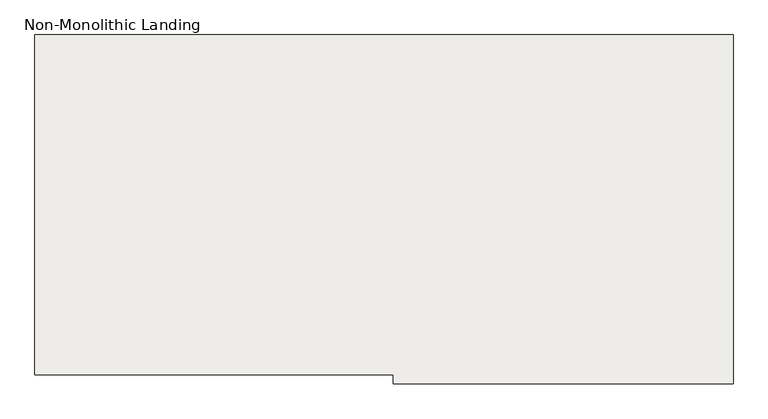
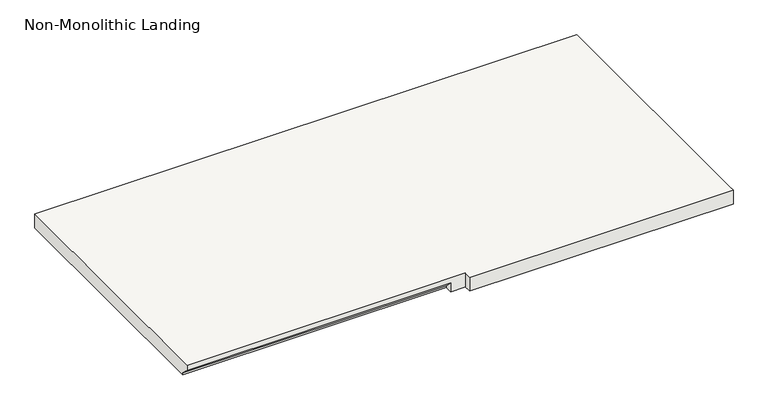
"""IFC4 building model written with IfcOpenShell, lengths in millimetres: slab geometry, Non-Monolithic Landing."""

from ifc_helpers import new_model, si_unit, origin, place, context, project, spatial, faceted_brep, source, transform, mapped, element, save


def non_monolithic_landing_f80fbcea(model_context):
    return source(origin(), model_context, "Body", "Brep", [
        faceted_brep([(282.3463194, 4459.6726898, 1352.55), (282.3463194, 4485.0726898, 1327.15), (1196.7463194, 4485.0726898, 1327.15), (1196.7463194, 4459.6726898, 1352.55), (1247.5463194, 4459.6726898, 1371.6), (1247.5463194, 4434.2726898, 1371.6), (2161.9463194, 4434.2726898, 1371.6), (2161.9463194, 4459.6726898, 1371.6), (2161.9463194, 5374.0726898, 1371.6), (282.3463194, 5374.0726898, 1371.6), (282.3463194, 4459.6726898, 1371.6), (1196.7463194, 4485.0726898, 1320.8), (282.3463194, 4485.0726898, 1320.8), (282.3463194, 5374.0726898, 1320.8), (2161.9463194, 5374.0726898, 1320.8), (2161.9463194, 4459.6726898, 1320.8), (2161.9463194, 4434.2726898, 1320.8), (1247.5463194, 4434.2726898, 1320.8), (1247.5463194, 4459.6726898, 1320.8), (1196.7463194, 4459.6726898, 1320.8)], [[[0, 1, 2, 3]], [[4, 5, 6, 7, 8, 9, 10]], [[11, 12, 13, 14, 15, 16, 17, 18, 19]], [[12, 11, 2, 1]], [[11, 19, 3, 2]], [[4, 10, 0, 3, 19, 18]], [[5, 4, 18, 17]], [[6, 5, 17, 16]], [[7, 6, 16, 15]], [[8, 7, 15, 14]], [[9, 8, 14, 13]], [[10, 9, 13, 12, 1, 0]]]),
    ])


if __name__ == "__main__":
    model = new_model("IFC4")
    model_context = context("Model", 3, world=origin())
    ifc_project = project(units=[si_unit("LENGTHUNIT", "METRE", prefix="MILLI")], contexts=[model_context])
    site = spatial("IfcSite", under=ifc_project)
    building = spatial("IfcBuilding", under=site)
    placement = place(None, origin())
    non_monolithic_landing_shape = non_monolithic_landing_f80fbcea(model_context)
    element("IfcSlab", 1, ObjectType="Non-Monolithic Landing", at=placement, inside=building, context=model_context, shape_type="MappedRepresentation", body=[
        mapped(non_monolithic_landing_shape, transform((0.0, 0.0, 0.0), x_axis=(1.0, 0.0, 0.0), y_axis=(0.0, 1.0, 0.0), z_axis=(0.0, 0.0, 1.0))),
    ])
    save(model, "model.ifc")
